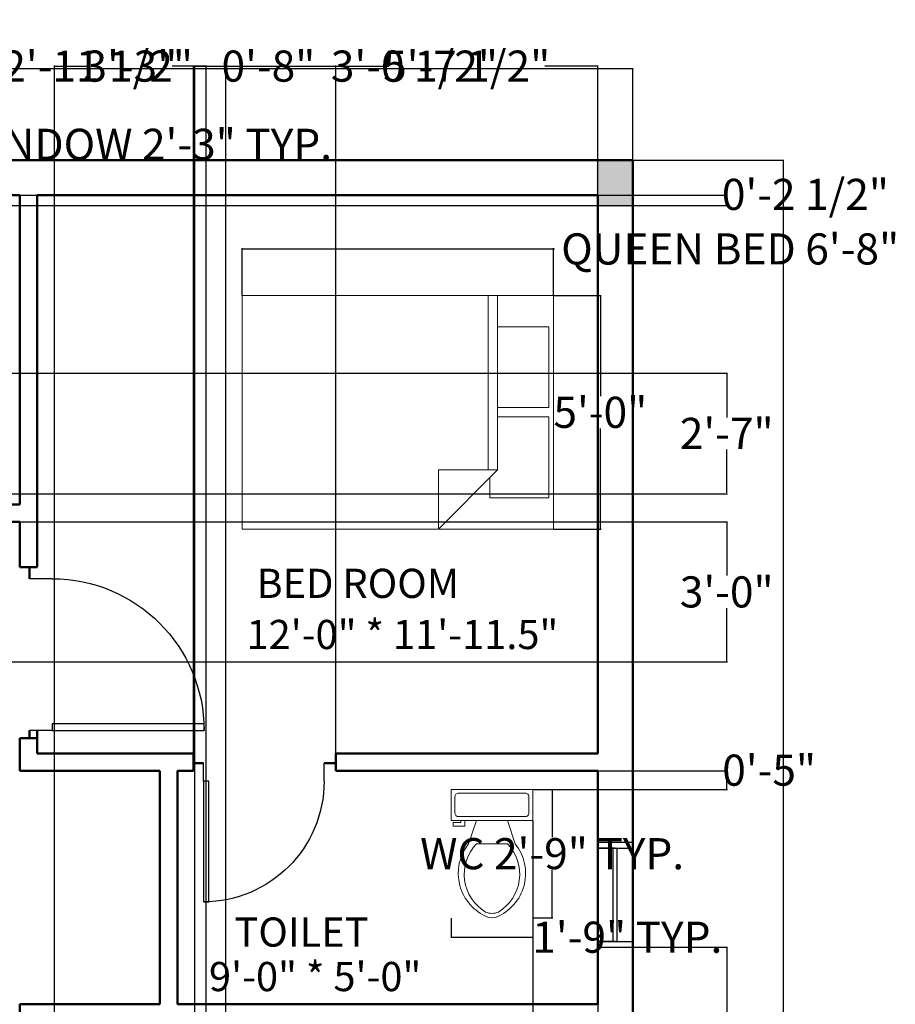
# Model space of a CAD drawing. Units: inches. Extents: x 9717 to 10218, y 17835 to 18358.
# Tile 4 of 4: x 9993 to 10218, y 18104 to 18358. Entities that reach past the tile are written whole.
import ezdxf

# ---------------------------------------------------------------- set-up
doc = ezdxf.new("R2010")
doc.units = ezdxf.units.IN
for name, color, linetype, lineweight in [('A-AREA-IDEN', 3, 'Continuous', 25), ('A-FLOR-FIXT', 2, 'Continuous', 18), ('COLUMN', 7, 'Continuous', 35), ('DIMENSIONS', 3, 'Continuous', 18), ('DOORS', 1, 'Continuous', 25), ('FURNITURES', 2, 'Continuous', 18), ('WALLS', 7, 'Continuous', 50), ('WINDOWS', 4, 'Continuous', 25)]:
    doc.layers.add(name, color=color, linetype=linetype, lineweight=lineweight)
doc.styles.get("Standard").update_dxf_attribs({"font": 'arial.ttf'})
doc.dimstyles.get("Standard").update_dxf_attribs({"dimtxt": 8, "dimasz": 0.18, "dimexe": 0.18, "dimexo": 0.0625, "dimgap": 0.09, "dimtad": 0, "dimtih": 1, "dimtoh": 1, "dimzin": 0, "dimdsep": 46, "dimlunit": 3, "dimtxsty": 'Standard', "dimcen": 0.09, "dimadec": 0, "dimazin": 0, "dimtfac": 1, "dimtofl": 0, "dimtmove": 0, "dimatfit": 3, "dimfxl": 1, "dimtolj": 1, "dimtzin": 0, "dimarcsym": 0})

# ---------------------------------------------------------------- blocks, each defined once
blk = doc.blocks.new('*U2')
for p, q in [((0, 0), (0, -6)), ((40, 0), (40, -6))]:
    blk.add_line(p, q)
blk.add_lwpolyline([(0, 0), (0, 40), (1.75, 40), (1.75, 0)], close=True)
blk.add_arc((0, 0), 40, 0, 90)
blk = doc.blocks.new('Bed - Queen')
for p, q in [((0, -80.00003), (0, 0)), ((0, 0), (59.99999, 0)), ((59.99999, 0), (59.99999, -80.00003)), ((7.99999, -1.2), (28.79998, -1.2)), ((7.99999, -14.4), (7.99999, -1.2)), ((28.79998, -1.2), (28.79998, -14.4)), ((31.19999, -1.2), (51.99999, -1.2)), ((31.19999, -14.4), (31.19999, -1.2)), ((51.99999, -1.2), (51.99999, -16.4)), ((0, -14.4), (44.8, -14.4)), ((59.99999, -29.6), (44.8, -14.4)), ((44.8, -14.4), (44.8, -29.6)), ((44.8, -16.8), (0, -16.8)), ((51.99999, -16.4), (46.79936, -16.4)), ((44.8, -29.6), (59.99999, -29.6)), ((59.99999, -80.00003), (0, -80.00003))]:
    blk.add_line(p, q)
blk = doc.blocks.new('Toilet - top')
for p, q in [((9.5, -6), (9.5, -2)), ((-10, -8.5), (-8, -8.5)), ((-10, -9.5), (-10, -8.5)), ((-7, -9.5), (-10, -9.5)), ((-8, -8.5), (-8, -8)), ((-7, -8), (-7, -9.5)), ((-4, -8), (-6, -14)), ((4, -8), (6, -14)), ((4, -14), (-4, -14))]:
    blk.add_line(p, q)
blk.add_lwpolyline([(10.5, -8), (10.5, 0), (-10.5, 0), (-10.5, -8)], close=True)
for points in [[(-9.5, -2), (-9.5, -6)], [(8.5, -1), (-8.5, -1)], [(-8.5, -7), (8.5, -7)]]:
    blk.add_lwpolyline(points)
for centre, radius, start, end in [((-8.62, -1.88), 0.884, 81.8699, 188.1301), ((8.62, -1.88), 0.884, 351.8699, 98.1301), ((-8.62, -6.12), 0.884, 171.8699, 278.1301), ((8.62, -6.12), 0.884, 261.8699, 8.1301), ((3.52, -21.58), 12.17, 141.4691, 247.9714), ((4.2, -21.82), 11.33, 136.3677, 238.9468), ((-3.52, -21.58), 12.17, 292.0284, 38.5307), ((-4.2, -21.82), 11.33, 301.053, 43.6321), ((0, -27.88), 4, 245.7318, 294.2682), ((0, -29), 4, 254.8605, 285.1395)]:
    blk.add_arc(centre, radius, start, end)
blk = doc.blocks.new('*D8')
at = {"layer": 'Defpoints', "color": 0, "transparency": 16777216}
for p in [(10150.76, 18344.92), (9772.76, 18321.49), (10150.76, 18321.49)]:
    blk.add_point(p, dxfattribs=at)
at = {"layer": 'DIMENSIONS', "color": 0, "lineweight": -2, "transparency": 16777216}
for p, q in [((9772.76, 18321.55), (9772.76, 18345.1)), ((9772.94, 18344.92), (9940.16, 18344.92)), ((10150.58, 18344.92), (9983.36, 18344.92)), ((10150.76, 18321.55), (10150.76, 18345.1))]:
    blk.add_line(p, q, dxfattribs=at)
at = {"layer": 'DIMENSIONS', "color": 0, "transparency": 16777216}
for points in [[(9772.94, 18344.95), (9772.94, 18344.89), (9772.76, 18344.92)], [(10150.58, 18344.95), (10150.58, 18344.89), (10150.76, 18344.92)]]:
    blk.add_solid(points, dxfattribs=at)
at = {"layer": 'DIMENSIONS', "color": 0, "transparency": 16777216, "insert": (9961.76, 18344.92), "char_height": 8, "attachment_point": 5}
blk.add_mtext('\\A1;31\'-6.00"', dxfattribs=at)
blk = doc.blocks.new('*D10')
at = {"layer": 'Defpoints', "color": 0, "transparency": 16777216}
for p in [(10150.76, 18321.49), (10150.76, 17871.49), (10189.42, 17871.49)]:
    blk.add_point(p, dxfattribs=at)
at = {"layer": 'DIMENSIONS', "color": 0, "lineweight": -2, "transparency": 16777216}
for p, q in [((10150.82, 18321.49), (10189.6, 18321.49)), ((10189.42, 18321.31), (10189.42, 18100.67)), ((10189.42, 17871.67), (10189.42, 18092.31)), ((10150.82, 17871.49), (10189.6, 17871.49))]:
    blk.add_line(p, q, dxfattribs=at)
at = {"layer": 'DIMENSIONS', "color": 0, "transparency": 16777216}
for points in [[(10189.39, 18321.31), (10189.45, 18321.31), (10189.42, 18321.49)], [(10189.39, 17871.67), (10189.45, 17871.67), (10189.42, 17871.49)]]:
    blk.add_solid(points, dxfattribs=at)
at = {"layer": 'DIMENSIONS', "color": 0, "transparency": 16777216, "insert": (10189.42, 18096.49), "char_height": 8, "attachment_point": 5}
blk.add_mtext('\\A1;37\'-6.00"', dxfattribs=at)
blk = doc.blocks.new('WIN-24IN')
for p, q in [((1.5, 9), (0, 9)), ((0, 9), (0, 0)), ((1.5, 4.5), (1.5, 9)), ((1.5, 9), (1.5, 0)), ((25.5, 4.5), (25.5, 9)), ((25.5, 9), (25.5, 0)), ((25.5, 9), (27, 9)), ((27, 9), (27, 0)), ((1.5, 5), (25.5, 5)), ((1.5, 4), (25.5, 4)), ((0, 0), (1.5, 0)), ((27, 0), (25.5, 0))]:
    blk.add_line(p, q)
blk = doc.blocks.new('COL-12X9IN')
h = blk.add_hatch(color=256)
h.dxf.hatch_style = 1
h.paths.add_polyline_path([(12, 0), (12, 9), (0, 9), (0, 0)])
blk = doc.blocks.new('*D18')
at = {"layer": 'Defpoints', "color": 0, "transparency": 16777216}
for p in [(9974.05, 18325.54), (9947.05, 18321.49), (9974.05, 18321.49)]:
    blk.add_point(p, dxfattribs=at)
at = {"layer": 'DIMENSIONS', "color": 0, "lineweight": -2, "transparency": 16777216}
for p, q in [((9947.05, 18321.55), (9947.05, 18325.72)), ((9947.23, 18325.54), (9973.87, 18325.54)), ((9974.05, 18321.55), (9974.05, 18325.72)), ((9974.05, 18325.54), (9974.23, 18325.54))]:
    blk.add_line(p, q, dxfattribs=at)
at = {"layer": 'DIMENSIONS', "color": 0, "transparency": 16777216}
for points in [[(9947.23, 18325.57), (9947.23, 18325.51), (9947.05, 18325.54)], [(9973.87, 18325.57), (9973.87, 18325.51), (9974.05, 18325.54)]]:
    blk.add_solid(points, dxfattribs=at)
at = {"layer": 'DIMENSIONS', "color": 0, "transparency": 16777216, "insert": (10024.94, 18325.54), "char_height": 8, "attachment_point": 5}
blk.add_mtext('\\A1;WINDOW 2\'-3" TYP.', dxfattribs=at)
blk = doc.blocks.new('*D24')
at = {"layer": 'Defpoints', "color": 0, "transparency": 16777216}
for p in [(10125.09, 18159.74), (10130.05, 18159.74), (10125.09, 18126.69)]:
    blk.add_point(p, dxfattribs=at)
at = {"layer": 'DIMENSIONS', "color": 0, "lineweight": -2, "transparency": 16777216}
for p, q in [((10125.16, 18159.74), (10130.23, 18159.74)), ((10130.05, 18159.56), (10130.05, 18147.44)), ((10130.05, 18126.87), (10130.05, 18138.99)), ((10125.16, 18126.69), (10130.23, 18126.69))]:
    blk.add_line(p, q, dxfattribs=at)
at = {"layer": 'DIMENSIONS', "color": 0, "transparency": 16777216}
for points in [[(10130.02, 18159.56), (10130.08, 18159.56), (10130.05, 18159.74)], [(10130.02, 18126.87), (10130.08, 18126.87), (10130.05, 18126.69)]]:
    blk.add_solid(points, dxfattribs=at)
at = {"layer": 'DIMENSIONS', "color": 0, "transparency": 16777216, "insert": (10130.05, 18143.21), "char_height": 8, "attachment_point": 5}
blk.add_mtext('\\A1;WC 2\'-9" TYP.', dxfattribs=at)
blk = doc.blocks.new('*D25')
at = {"layer": 'Defpoints', "color": 0, "transparency": 16777216}
for p in [(10104.09, 18126.69), (10125.09, 18126.69), (10125.09, 18121.73)]:
    blk.add_point(p, dxfattribs=at)
at = {"layer": 'DIMENSIONS', "color": 0, "lineweight": -2, "transparency": 16777216}
for p, q in [((10104.09, 18126.63), (10104.09, 18121.55)), ((10125.09, 18126.63), (10125.09, 18121.55)), ((10104.27, 18121.73), (10124.91, 18121.73)), ((10125.09, 18121.73), (10125.27, 18121.73))]:
    blk.add_line(p, q, dxfattribs=at)
at = {"layer": 'DIMENSIONS', "color": 0, "transparency": 16777216}
for points in [[(10104.27, 18121.76), (10104.27, 18121.7), (10104.09, 18121.73)], [(10124.91, 18121.76), (10124.91, 18121.7), (10125.09, 18121.73)]]:
    blk.add_solid(points, dxfattribs=at)
at = {"layer": 'DIMENSIONS', "color": 0, "transparency": 16777216, "insert": (10149.37, 18121.73), "char_height": 8, "attachment_point": 5}
blk.add_mtext('\\A1;1\'-9" TYP.', dxfattribs=at)
blk = doc.blocks.new('*D26')
at = {"layer": 'Defpoints', "color": 0, "transparency": 16777216}
for p in [(10130.44, 18298.65), (10050.44, 18286.65), (10130.44, 18286.65)]:
    blk.add_point(p, dxfattribs=at)
at = {"layer": 'DIMENSIONS', "color": 0, "lineweight": -2, "transparency": 16777216}
for p, q in [((10050.44, 18286.71), (10050.44, 18298.83)), ((10050.62, 18298.65), (10130.26, 18298.65)), ((10130.44, 18286.71), (10130.44, 18298.83)), ((10130.44, 18298.65), (10130.62, 18298.65))]:
    blk.add_line(p, q, dxfattribs=at)
at = {"layer": 'DIMENSIONS', "color": 0, "transparency": 16777216}
for points in [[(10050.62, 18298.68), (10050.62, 18298.62), (10050.44, 18298.65)], [(10130.26, 18298.68), (10130.26, 18298.62), (10130.44, 18298.65)]]:
    blk.add_solid(points, dxfattribs=at)
at = {"layer": 'DIMENSIONS', "color": 0, "transparency": 16777216, "insert": (10175.8, 18298.65), "char_height": 8, "attachment_point": 5}
blk.add_mtext('\\A1;QUEEN BED 6\'-8"', dxfattribs=at)
blk = doc.blocks.new('*D27')
at = {"layer": 'Defpoints', "color": 0, "transparency": 16777216}
for p in [(10130.44, 18286.65), (10130.44, 18226.65), (10142.44, 18226.65)]:
    blk.add_point(p, dxfattribs=at)
at = {"layer": 'DIMENSIONS', "color": 0, "lineweight": -2, "transparency": 16777216}
for p, q in [((10130.51, 18286.65), (10142.62, 18286.65)), ((10142.44, 18286.47), (10142.44, 18260.83)), ((10142.44, 18226.83), (10142.44, 18252.48)), ((10130.51, 18226.65), (10142.62, 18226.65))]:
    blk.add_line(p, q, dxfattribs=at)
at = {"layer": 'DIMENSIONS', "color": 0, "transparency": 16777216}
for points in [[(10142.41, 18286.47), (10142.47, 18286.47), (10142.44, 18286.65)], [(10142.41, 18226.83), (10142.47, 18226.83), (10142.44, 18226.65)]]:
    blk.add_solid(points, dxfattribs=at)
at = {"layer": 'DIMENSIONS', "color": 0, "transparency": 16777216, "insert": (10142.44, 18256.65), "char_height": 8, "attachment_point": 5}
blk.add_mtext('\\A1;5\'-0"', dxfattribs=at)
blk = doc.blocks.new('*D39')
at = {"layer": 'Defpoints', "color": 0, "transparency": 16777216}
for p in [(10046.260349, 18345.641492), (10038.260349, 17915.241492), (10046.260349, 17915.241492)]:
    blk.add_point(p, dxfattribs=at)
at = {"layer": 'DIMENSIONS', "color": 0, "lineweight": -2, "transparency": 16777216}
for p, q in [((10038.260349, 17915.303992), (10038.260349, 18345.821492)), ((10046.260349, 17915.303992), (10046.260349, 18345.821492)), ((10038.440349, 18345.641492), (10046.080349, 18345.641492)), ((10046.260349, 18345.641492), (10046.440349, 18345.641492))]:
    blk.add_line(p, q, dxfattribs=at)
at = {"layer": 'DIMENSIONS', "color": 0, "transparency": 16777216}
for points in [[(10038.440349, 18345.671492), (10038.440349, 18345.611492), (10038.260349, 18345.641492)], [(10046.080349, 18345.671492), (10046.080349, 18345.611492), (10046.260349, 18345.641492)]]:
    blk.add_solid(points, dxfattribs=at)
at = {"layer": 'DIMENSIONS', "color": 0, "transparency": 16777216, "insert": (10057.163364, 18345.641492), "char_height": 8, "attachment_point": 5}
blk.add_mtext('\\A1;0\'-8"', dxfattribs=at)
blk = doc.blocks.new('*D47')
at = {"layer": 'Defpoints', "color": 0, "transparency": 16777216}
for p in [(10150.76, 18119.16), (10174.91, 18119.16), (10150.76, 18064.34)]:
    blk.add_point(p, dxfattribs=at)
at = {"layer": 'DIMENSIONS', "color": 0, "lineweight": -2, "transparency": 16777216}
for p, q in [((10150.82, 18119.16), (10175.09, 18119.16)), ((10174.91, 18118.98), (10174.91, 18095.84)), ((10174.91, 18064.52), (10174.91, 18087.66)), ((10150.82, 18064.34), (10175.09, 18064.34))]:
    blk.add_line(p, q, dxfattribs=at)
at = {"layer": 'DIMENSIONS', "color": 0, "transparency": 16777216}
for points in [[(10174.88, 18118.98), (10174.94, 18118.98), (10174.91, 18119.16)], [(10174.88, 18064.52), (10174.94, 18064.52), (10174.91, 18064.34)]]:
    blk.add_solid(points, dxfattribs=at)
at = {"layer": 'DIMENSIONS', "color": 0, "transparency": 16777216, "insert": (10174.91, 18091.75), "char_height": 8, "attachment_point": 5}
blk.add_mtext('\\A1;4\'-7"', dxfattribs=at)
blk = doc.blocks.new('*D50')
at = {"layer": 'Defpoints', "color": 0, "transparency": 16777216}
for p in [(9930.26, 18228.49), (10174.91, 18228.49), (9930.26, 18192.49)]:
    blk.add_point(p, dxfattribs=at)
at = {"layer": 'DIMENSIONS', "color": 0, "lineweight": -2, "transparency": 16777216}
for p, q in [((9930.32, 18228.49), (10175.09, 18228.49)), ((10174.91, 18228.31), (10174.91, 18214.67)), ((10174.91, 18192.67), (10174.91, 18206.31)), ((9930.32, 18192.49), (10175.09, 18192.49))]:
    blk.add_line(p, q, dxfattribs=at)
at = {"layer": 'DIMENSIONS', "color": 0, "transparency": 16777216}
for points in [[(10174.88, 18228.31), (10174.94, 18228.31), (10174.91, 18228.49)], [(10174.88, 18192.67), (10174.94, 18192.67), (10174.91, 18192.49)]]:
    blk.add_solid(points, dxfattribs=at)
at = {"layer": 'DIMENSIONS', "color": 0, "transparency": 16777216, "insert": (10174.91, 18210.49), "char_height": 8, "attachment_point": 5}
blk.add_mtext('\\A1;3\'-0"', dxfattribs=at)
blk = doc.blocks.new('*D51')
at = {"layer": 'Defpoints', "color": 0, "transparency": 16777216}
for p in [(9989.89, 18345.64), (9954.27, 18232.99), (9989.89, 18232.99)]:
    blk.add_point(p, dxfattribs=at)
at = {"layer": 'DIMENSIONS', "color": 0, "lineweight": -2, "transparency": 16777216}
for p, q in [((9954.27, 18233.05), (9954.27, 18345.82)), ((9989.89, 18233.05), (9989.89, 18345.82)), ((9954.45, 18345.64), (9989.71, 18345.64)), ((9989.89, 18345.64), (9990.07, 18345.64))]:
    blk.add_line(p, q, dxfattribs=at)
at = {"layer": 'DIMENSIONS', "color": 0, "transparency": 16777216}
for points in [[(9954.45, 18345.67), (9954.45, 18345.61), (9954.27, 18345.64)], [(9989.71, 18345.67), (9989.71, 18345.61), (9989.89, 18345.64)]]:
    blk.add_solid(points, dxfattribs=at)
at = {"layer": 'DIMENSIONS', "color": 0, "transparency": 16777216, "insert": (10013.29, 18345.64), "char_height": 8, "attachment_point": 5}
blk.add_mtext('\\A1;2\'-11 1/2"', dxfattribs=at)
blk = doc.blocks.new('*D53')
at = {"layer": 'Defpoints', "color": 0, "transparency": 16777216}
for p in [(10074.45, 18345.64), (10037.94, 18168.99), (10074.45, 18168.99)]:
    blk.add_point(p, dxfattribs=at)
at = {"layer": 'DIMENSIONS', "color": 0, "lineweight": -2, "transparency": 16777216}
for p, q in [((10037.94, 18169.05), (10037.94, 18345.82)), ((10074.45, 18169.05), (10074.45, 18345.82)), ((10038.12, 18345.64), (10074.27, 18345.64)), ((10074.45, 18345.64), (10074.63, 18345.64))]:
    blk.add_line(p, q, dxfattribs=at)
at = {"layer": 'DIMENSIONS', "color": 0, "transparency": 16777216}
for points in [[(10038.12, 18345.67), (10038.12, 18345.61), (10037.94, 18345.64)], [(10074.27, 18345.67), (10074.27, 18345.61), (10074.45, 18345.64)]]:
    blk.add_solid(points, dxfattribs=at)
at = {"layer": 'DIMENSIONS', "color": 0, "transparency": 16777216, "insert": (10094.67, 18345.64), "char_height": 8, "attachment_point": 5}
blk.add_mtext('\\A1;3\'-0 1/2"', dxfattribs=at)
blk = doc.blocks.new('*D56')
at = {"layer": 'Defpoints', "color": 0, "transparency": 16777216}
for p in [(9986.65, 18266.74), (10174.91, 18266.74), (9986.65, 18235.74)]:
    blk.add_point(p, dxfattribs=at)
at = {"layer": 'DIMENSIONS', "color": 0, "lineweight": -2, "transparency": 16777216}
for p, q in [((9986.71, 18266.74), (10175.09, 18266.74)), ((10174.91, 18266.56), (10174.91, 18255.34)), ((10174.91, 18235.92), (10174.91, 18247.13)), ((9986.71, 18235.74), (10175.09, 18235.74))]:
    blk.add_line(p, q, dxfattribs=at)
at = {"layer": 'DIMENSIONS', "color": 0, "transparency": 16777216}
for points in [[(10174.88, 18266.56), (10174.94, 18266.56), (10174.91, 18266.74)], [(10174.88, 18235.92), (10174.94, 18235.92), (10174.91, 18235.74)]]:
    blk.add_solid(points, dxfattribs=at)
at = {"layer": 'DIMENSIONS', "color": 0, "transparency": 16777216, "insert": (10174.91, 18251.24), "char_height": 8, "attachment_point": 5}
blk.add_mtext('\\A1;2\'-7"', dxfattribs=at)
blk = doc.blocks.new('*D57')
at = {"layer": 'Defpoints', "color": 0, "transparency": 16777216}
for p in [(10041.19, 18345.64), (10002.19, 17978.77), (10041.19, 17978.77)]:
    blk.add_point(p, dxfattribs=at)
at = {"layer": 'DIMENSIONS', "color": 0, "lineweight": -2, "transparency": 16777216}
for p, q in [((10002.19, 17978.83), (10002.19, 18345.82)), ((10041.19, 17978.83), (10041.19, 18345.82)), ((10002.37, 18345.64), (10010.97, 18345.64)), ((10041.01, 18345.64), (10032.41, 18345.64))]:
    blk.add_line(p, q, dxfattribs=at)
at = {"layer": 'DIMENSIONS', "color": 0, "transparency": 16777216}
for points in [[(10002.37, 18345.67), (10002.37, 18345.61), (10002.19, 18345.64)], [(10041.01, 18345.67), (10041.01, 18345.61), (10041.19, 18345.64)]]:
    blk.add_solid(points, dxfattribs=at)
at = {"layer": 'DIMENSIONS', "color": 0, "transparency": 16777216, "insert": (10021.69, 18345.64), "char_height": 8, "attachment_point": 5}
blk.add_mtext('\\A1;3\'-3"', dxfattribs=at)
blk = doc.blocks.new('*D59')
at = {"layer": 'Defpoints', "color": 0, "transparency": 16777216}
for p in [(10141.76, 18345.64), (10074.45, 18168.99), (10141.76, 18168.99)]:
    blk.add_point(p, dxfattribs=at)
at = {"layer": 'DIMENSIONS', "color": 0, "lineweight": -2, "transparency": 16777216}
for p, q in [((10074.45, 18169.05), (10074.45, 18345.82)), ((10141.76, 18169.05), (10141.76, 18345.82)), ((10074.63, 18345.64), (10088.06, 18345.64)), ((10141.58, 18345.64), (10128.15, 18345.64))]:
    blk.add_line(p, q, dxfattribs=at)
at = {"layer": 'DIMENSIONS', "color": 0, "transparency": 16777216}
for points in [[(10074.63, 18345.67), (10074.63, 18345.61), (10074.45, 18345.64)], [(10141.58, 18345.67), (10141.58, 18345.61), (10141.76, 18345.64)]]:
    blk.add_solid(points, dxfattribs=at)
at = {"layer": 'DIMENSIONS', "color": 0, "transparency": 16777216, "insert": (10108.1, 18345.64), "char_height": 8, "attachment_point": 5}
blk.add_mtext('\\A1;5\'-7 1/2"', dxfattribs=at)
blk = doc.blocks.new('*D65')
at = {"layer": 'Defpoints', "color": 0, "transparency": 16777216}
for p in [(10125.09, 18151.74), (10141.76, 18146.16), (10141.76, 17847.34)]:
    blk.add_point(p, dxfattribs=at)
at = {"layer": 'DIMENSIONS', "color": 0, "lineweight": -2, "transparency": 16777216}
for p, q in [((10125.09, 18151.67), (10125.09, 17847.16)), ((10141.76, 18146.09), (10141.76, 17847.16)), ((10125.27, 17847.34), (10141.58, 17847.34)), ((10141.76, 17847.34), (10141.94, 17847.34))]:
    blk.add_line(p, q, dxfattribs=at)
at = {"layer": 'DIMENSIONS', "color": 0, "transparency": 16777216}
for points in [[(10125.27, 17847.37), (10125.27, 17847.31), (10125.09, 17847.34)], [(10141.58, 17847.37), (10141.58, 17847.31), (10141.76, 17847.34)]]:
    blk.add_solid(points, dxfattribs=at)
at = {"layer": 'DIMENSIONS', "color": 0, "transparency": 16777216, "insert": (10161.61, 17847.34), "char_height": 8, "attachment_point": 5}
blk.add_mtext('\\A1;1\'-4 1/2"', dxfattribs=at)
blk = doc.blocks.new('*D66')
at = {"layer": 'Defpoints', "color": 0, "transparency": 16777216}
for p in [(10141.760349, 18164.491492), (10174.910349, 18164.491492), (10125.094777, 18159.73745)]:
    blk.add_point(p, dxfattribs=at)
at = {"layer": 'DIMENSIONS', "color": 0, "lineweight": -2, "transparency": 16777216}
for p, q in [((10141.822849, 18164.491492), (10175.090349, 18164.491492)), ((10174.910349, 18164.491492), (10174.910349, 18164.671492)), ((10174.910349, 18164.671492), (10175.090349, 18164.671492)), ((10174.910349, 18159.91745), (10174.910349, 18164.311492)), ((10125.157277, 18159.73745), (10175.090349, 18159.73745))]:
    blk.add_line(p, q, dxfattribs=at)
at = {"layer": 'DIMENSIONS', "color": 0, "transparency": 16777216}
for points in [[(10174.880349, 18164.311492), (10174.940349, 18164.311492), (10174.910349, 18164.491492)], [(10174.880349, 18159.91745), (10174.940349, 18159.91745), (10174.910349, 18159.73745)]]:
    blk.add_solid(points, dxfattribs=at)
at = {"layer": 'DIMENSIONS', "color": 0, "transparency": 16777216, "insert": (10185.813364, 18164.671492), "char_height": 8, "attachment_point": 5}
blk.add_mtext('\\A1;0\'-5"', dxfattribs=at)
blk = doc.blocks.new('*D67')
at = {"layer": 'Defpoints', "color": 0, "transparency": 16777216}
for p in [(9974.05, 18312.49), (10174.91, 18312.49), (9972.25, 18309.85)]:
    blk.add_point(p, dxfattribs=at)
at = {"layer": 'DIMENSIONS', "color": 0, "lineweight": -2, "transparency": 16777216}
for p, q in [((9974.12, 18312.49), (10175.09, 18312.49)), ((10174.91, 18312.49), (10174.91, 18312.67)), ((10174.91, 18312.67), (10175.09, 18312.67)), ((10174.91, 18310.03), (10174.91, 18312.31)), ((9972.31, 18309.85), (10175.09, 18309.85))]:
    blk.add_line(p, q, dxfattribs=at)
at = {"layer": 'DIMENSIONS', "color": 0, "transparency": 16777216}
for points in [[(10174.88, 18312.31), (10174.94, 18312.31), (10174.91, 18312.49)], [(10174.88, 18310.03), (10174.94, 18310.03), (10174.91, 18309.85)]]:
    blk.add_solid(points, dxfattribs=at)
at = {"layer": 'DIMENSIONS', "color": 0, "transparency": 16777216, "insert": (10195.13, 18312.67), "char_height": 8, "attachment_point": 5}
blk.add_mtext('\\A1;0\'-2 1/2"', dxfattribs=at)

msp = doc.modelspace()

# ---------------------------------------------------------------- linework, layer by layer
at = {"layer": 'WALLS'}
for p, q in [((9930.26, 18312.491), (9993.26, 18312.491)), ((9993.26, 18232.991), (9993.26, 18312.491)), ((9997.76, 18312.491), (10141.76, 18312.491)), ((9997.76, 18216.874), (9997.76, 18312.491)), ((10141.76, 18312.491), (10141.76, 18168.991)), ((9989.894, 18232.991), (9993.26, 18232.991)), ((9989.894, 18228.491), (9993.26, 18228.491)), ((9993.26, 18216.874), (9993.26, 18228.491)), ((9997.76, 18216.874), (9993.26, 18216.874)), ((9995.786, 18213.872), (9995.786, 18216.874)), ((9995.786, 18174.872), (9995.786, 18172.923)), ((9997.76, 18168.991), (9997.76, 18174.872)), ((9993.26, 18164.491), (9993.26, 18172.923)), ((9993.26, 18172.923), (9997.76, 18172.923)), ((9997.76, 18168.991), (10037.937, 18168.991)), ((10037.937, 18168.991), (10037.937, 18164.491)), ((10074.447, 18164.491), (10074.447, 18168.991)), ((10074.447, 18168.991), (10141.76, 18168.991)), ((10040.46, 18166.476), (10037.937, 18166.476)), ((10071.46, 18166.476), (10074.447, 18166.476)), ((9993.26, 18164.491), (10029.26, 18164.491)), ((10029.26, 18164.491), (10029.26, 18104.491)), ((10033.76, 18164.491), (10033.76, 18104.491)), ((10033.76, 18164.491), (10037.937, 18164.491)), ((10074.447, 18164.491), (10141.76, 18164.491)), ((10141.76, 18164.491), (10141.76, 18104.491)), ((9993.26, 18104.491), (10029.26, 18104.491)), ((9993.26, 18104.491), (9993.26, 18020.621)), ((10033.76, 18104.491), (10141.76, 18104.491))]:
    msp.add_line(p, q, dxfattribs=at)
msp.add_lwpolyline([(9867.276, 17961.491), (9772.76, 17961.491), (9772.76, 18321.491), (10150.76, 18321.491), (10150.76, 17961.491)], dxfattribs=at)

# ---------------------------------------------------------------- block references
at = {"layer": 'A-FLOR-FIXT'}
msp.add_blockref('Toilet - top', (10114.595, 18159.737), dxfattribs=at)
at = {"layer": 'COLUMN', "rotation": 269.9999999999907}
msp.add_blockref('COL-12X9IN', (10141.531, 18321.492), dxfattribs=at)
at = {"layer": 'DOORS'}
for p, xscale, yscale, zscale, rotation in [((10001.636, 18174.872), -0.975, 0.975, 0.975, 270), ((10040.46, 18161.826), -0.775, 0.775, 0.775, 180)]:
    msp.add_blockref('*U2', p, dxfattribs=dict(at, xscale=xscale, yscale=yscale, zscale=zscale, rotation=rotation))
at = {"layer": 'FURNITURES', "rotation": 270}
msp.add_blockref('Bed - Queen', (10130.443, 18286.65), dxfattribs=at)
at = {"layer": 'WINDOWS', "rotation": 90.00000000000003}
msp.add_blockref('WIN-24IN', (10150.761, 18119.155), dxfattribs=at)

# ---------------------------------------------------------------- texts
at = {"layer": 'A-AREA-IDEN'}
for s, p in [('BED ROOM', (10054.097, 18208.943)), ('12\'-0" * 11\'-11.5"', (10051.525, 18195.798)), ('TOILET ', (10048.45, 18119.312)), ('9\'-0" * 5\'-0"', (10041.892, 18107.876))]:
    msp.add_text(s, height=7.5, dxfattribs=at).set_placement(p)

# ---------------------------------------------------------------- dimensions: what is measured, and where the dimension line sits
at = {"layer": 'DIMENSIONS'}
for base, p1, p2, override, picture, middle in [((9989.894, 18345.641), (9954.275, 18232.991), (9989.894, 18232.991), {"dimdec": 1, "dimlfac": 1, "dimrnd": 0, "dimzin": 1, "dimdsep": 46, "dimlunit": 4, "dimfrac": 2}, '*D51', (10013.293, 18345.641)), ((10074.447, 18345.641), (10037.937, 18168.991), (10074.447, 18168.991), {"dimdec": 1, "dimlfac": 1, "dimrnd": 0, "dimzin": 1, "dimdsep": 46, "dimlunit": 4, "dimfrac": 2}, '*D53', (10094.668, 18345.641)), ((10141.76, 18345.641), (10074.447, 18168.991), (10141.76, 18168.991), {"dimdec": 1, "dimlfac": 1, "dimrnd": 0, "dimzin": 1, "dimdsep": 46, "dimlunit": 4, "dimfrac": 2}, '*D59', (10108.104, 18345.641)), ((10041.187, 18345.641), (10002.187, 17978.769), (10041.187, 17978.769), {"dimdec": 1, "dimlfac": 1, "dimrnd": 0, "dimzin": 1, "dimdsep": 46, "dimlunit": 4, "dimfrac": 2}, '*D57', (10021.687, 18345.641)), ((10046.26, 18345.641), (10038.26, 17915.241), (10046.26, 17915.241), {"dimdec": 1, "dimlfac": 1, "dimrnd": 0, "dimzin": 1, "dimdsep": 46, "dimlunit": 4, "dimfrac": 2}, '*D39', (10057.163, 18345.641)), ((10150.76, 18344.922), (9772.76, 18321.491), (10150.76, 18321.491), {"dimclrd": 0, "dimclre": 0, "dimclrt": 0}, '*D8', (9961.76, 18344.922)), ((10141.76, 17847.341), (10125.095, 18151.737), (10141.76, 18146.155), {"dimdec": 1, "dimlfac": 1, "dimrnd": 0, "dimzin": 1, "dimdsep": 46, "dimlunit": 4, "dimfrac": 2}, '*D65', (10161.607, 17847.341))]:
    dim = msp.add_linear_dim(base=base, p1=p1, p2=p2, dimstyle='Standard', override=override, dxfattribs=at)
    dim.commit()
    dim.dimension.update_dxf_attribs({"geometry": picture, "text_midpoint": middle})
for base, p1, p2, text, picture, middle in [((9974.053, 18325.541), (9947.053, 18321.491), (9974.053, 18321.491), 'WINDOW <> TYP.', '*D18', (10024.939, 18325.541)), ((10130.443, 18298.65), (10050.443, 18286.65), (10130.443, 18286.65), 'QUEEN BED <>', '*D26', (10175.804, 18298.65)), ((10125.095, 18121.734), (10104.095, 18126.691), (10125.095, 18126.691), '<> TYP.', '*D25', (10149.37, 18121.734))]:
    dim = msp.add_linear_dim(base=base, p1=p1, p2=p2, text=text, dimstyle='Standard', override={"dimdec": 1, "dimlfac": 1, "dimrnd": 0, "dimzin": 1, "dimdsep": 46, "dimlunit": 4, "dimfrac": 2}, dxfattribs=at)
    dim.commit()
    dim.dimension.update_dxf_attribs({"geometry": picture, "text_midpoint": middle})
for base, p1, p2, angle, override, picture, middle in [((10174.91, 18312.491), (9972.246, 18309.847), (9974.053, 18312.491), 90, {"dimdec": 1, "dimlfac": 1, "dimrnd": 0, "dimzin": 1, "dimdsep": 46, "dimlunit": 4, "dimfrac": 2}, '*D67', (10195.134, 18312.671)), ((10189.422, 17871.491), (10150.76, 18321.491), (10150.76, 17871.491), 90, {"dimclrd": 0, "dimclre": 0, "dimclrt": 0}, '*D10', (10189.422, 18096.491)), ((10142.443, 18226.65), (10130.443, 18286.65), (10130.443, 18226.65), 270, {"dimdec": 1, "dimlfac": 1, "dimrnd": 0, "dimzin": 1, "dimdsep": 46, "dimlunit": 4, "dimfrac": 2}, '*D27', (10142.443, 18256.65)), ((10174.91, 18266.736), (9986.649, 18235.736), (9986.649, 18266.736), 90, {"dimdec": 1, "dimlfac": 1, "dimrnd": 0, "dimzin": 1, "dimdsep": 46, "dimlunit": 4, "dimfrac": 2}, '*D56', (10174.91, 18251.236)), ((10174.91, 18228.491), (9930.26, 18192.491), (9930.26, 18228.491), 90, {"dimdec": 1, "dimlfac": 1, "dimrnd": 0, "dimzin": 1, "dimdsep": 46, "dimlunit": 4, "dimfrac": 2}, '*D50', (10174.91, 18210.491)), ((10174.91, 18164.491), (10125.095, 18159.737), (10141.76, 18164.491), 90, {"dimdec": 1, "dimlfac": 1, "dimrnd": 0, "dimzin": 1, "dimdsep": 46, "dimlunit": 4, "dimfrac": 2}, '*D66', (10185.813, 18164.671)), ((10174.91, 18119.155), (10150.76, 18064.339), (10150.76, 18119.155), 90, {"dimdec": 1, "dimlfac": 1, "dimrnd": 0, "dimzin": 1, "dimdsep": 46, "dimlunit": 4, "dimfrac": 2}, '*D47', (10174.91, 18091.747))]:
    dim = msp.add_linear_dim(base=base, p1=p1, p2=p2, angle=angle, dimstyle='Standard', override=override, dxfattribs=at)
    dim.commit()
    dim.dimension.update_dxf_attribs({"geometry": picture, "text_midpoint": middle})
dim = msp.add_linear_dim(base=(10130.052, 18159.737), p1=(10125.095, 18126.691), p2=(10125.095, 18159.737), angle=90, text='WC <> TYP.', dimstyle='Standard', override={"dimdec": 1, "dimlfac": 1, "dimrnd": 0, "dimzin": 1, "dimdsep": 46, "dimlunit": 4, "dimfrac": 2}, dxfattribs=at)
dim.commit()
dim.dimension.update_dxf_attribs({"geometry": '*D24', "text_midpoint": (10130.052, 18143.214)})

doc.saveas('drawing.dxf')
